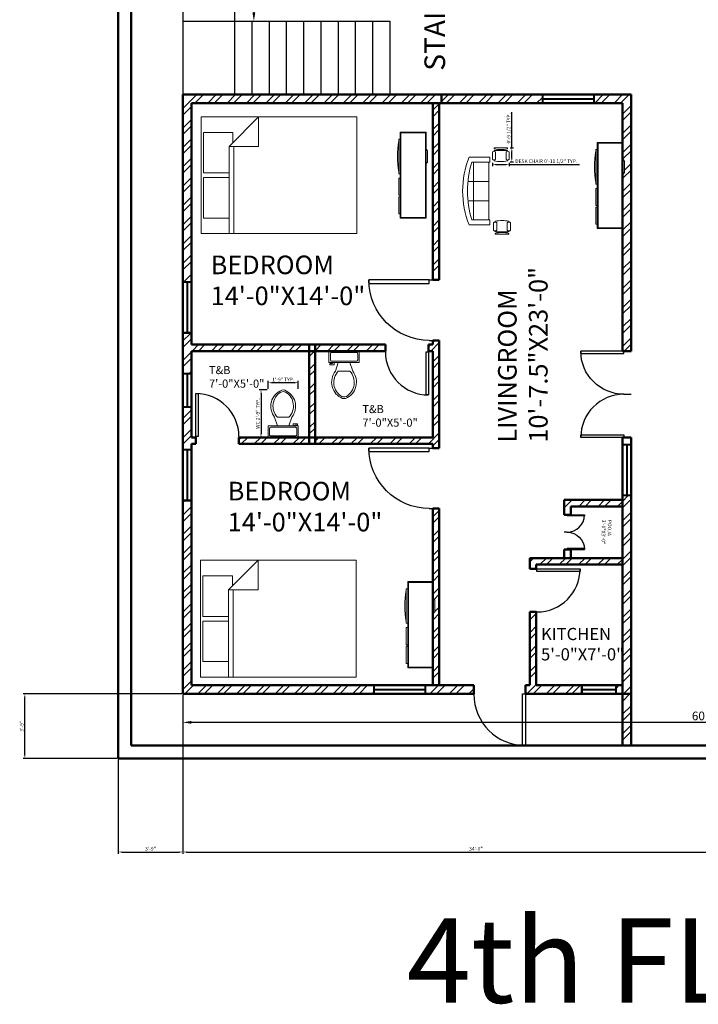
# Model space of a CAD drawing. Units: inches. Extents: x -12550 to 6516, y 1273 to 18700.
# Tile 16 of 19: x 5571 to 6043, y 1273 to 1958. Entities that reach past the tile are written whole.
import ezdxf

# ---------------------------------------------------------------- set-up
doc = ezdxf.new("R2010")
doc.units = ezdxf.units.IN
for name, color, linetype, lineweight in [('A-ANNO-DIMS', 2, 'Continuous', 18), ('A-ANNO-TEXT', 7, 'Continuous', 25), ('A-AREA-IDEN', 1, 'Continuous', 18), ('A-DOOR', 5, 'Continuous', 25), ('A-FLOR-STRS', 6, 'Continuous', 25), ('A-FURN', 8, 'Continuous', 18), ('A-GLAZ', 3, 'Continuous', 25), ('A-WALL', 7, 'Continuous', 50), ('A-WALL-PATT', 8, 'Continuous', 13)]:
    doc.layers.add(name, color=color, linetype=linetype, lineweight=lineweight)
doc.styles.get("Standard").update_dxf_attribs({"font": 'arial.ttf'})
doc.dimstyles.new('ISO-25', dxfattribs={"dimtxt": 2.5, "dimasz": 2.5, "dimexe": 1.25, "dimexo": 0.625, "dimtad": 1, "dimlunit": 4, "dimtxsty": 'Standard', "dimcen": 2.5, "dimadec": 0, "dimazin": 0, "dimtfac": 1, "dimtmove": 0, "dimatfit": 3, "dimfxl": 1, "dimarcsym": 0})
pattern_1 = [(45, (3666.851, 0), (-6.735192, 6.735192), []), (45, (3671.341, 0), (-6.735192, 6.735192), [])]

# ---------------------------------------------------------------- blocks, each defined once
blk = doc.blocks.new('*U2')
for p, q in [((0, 0), (0, -5)), ((30, 0), (30, -5))]:
    blk.add_line(p, q)
blk.add_lwpolyline([(0, 0), (0, 30), (1.75, 30), (1.75, 0)], close=True)
blk.add_arc((0, 0), 30, 0, 90)
blk = doc.blocks.new('Bed - Queen')
for p, q in [((0, -80.00003), (0, 0)), ((0, 0), (59.99999, 0)), ((59.99999, 0), (59.99999, -80.00003)), ((7.99999, -1.2), (28.79998, -1.2)), ((7.99999, -14.4), (7.99999, -1.2)), ((28.79998, -1.2), (28.79998, -14.4)), ((31.19999, -1.2), (51.99999, -1.2)), ((31.19999, -14.4), (31.19999, -1.2)), ((51.99999, -1.2), (51.99999, -16.4)), ((0, -14.4), (44.8, -14.4)), ((59.99999, -29.6), (44.8, -14.4)), ((44.8, -14.4), (44.8, -29.6)), ((44.8, -16.8), (0, -16.8)), ((51.99999, -16.4), (46.79936, -16.4)), ((44.8, -29.6), (59.99999, -29.6)), ((59.99999, -80.00003), (0, -80.00003))]:
    blk.add_line(p, q)
blk = doc.blocks.new('Toilet - top')
for p, q in [((9.5, -6), (9.5, -2)), ((-10, -8.5), (-8, -8.5)), ((-10, -9.5), (-10, -8.5)), ((-7, -9.5), (-10, -9.5)), ((-8, -8.5), (-8, -8)), ((-7, -8), (-7, -9.5)), ((-4, -8), (-6, -14)), ((4, -8), (6, -14)), ((4, -14), (-4, -14))]:
    blk.add_line(p, q)
blk.add_lwpolyline([(10.5, -8), (10.5, 0), (-10.5, 0), (-10.5, -8)], close=True)
for points in [[(-9.5, -2), (-9.5, -6)], [(8.5, -1), (-8.5, -1)], [(-8.5, -7), (8.5, -7)]]:
    blk.add_lwpolyline(points)
for centre, radius, start, end in [((-8.62, -1.88), 0.884, 81.8699, 188.1301), ((-8.62, -6.12), 0.884, 171.8699, 278.1301), ((8.62, -1.88), 0.884, 351.8699, 98.1301), ((8.62, -6.12), 0.884, 261.8699, 8.1301), ((3.52, -21.58), 12.17, 141.46911, 247.97143), ((4.2, -21.82), 11.33, 136.36773, 238.94682), ((-3.52, -21.58), 12.17, 292.02843, 38.53071), ((-4.2, -21.82), 11.33, 301.05301, 43.63209), ((0, -27.88), 4, 245.73182, 294.26817), ((0, -29), 4, 254.86053, 285.13947)]:
    blk.add_arc(centre, radius, start, end)
blk = doc.blocks.new('Entertainment Center')
for p, q in [((-4, 0), (-5, -1)), ((4, 0), (-4, 0)), ((5, -1), (4, 0)), ((-17, -19), (-17, -1)), ((-17, -1), (43, -1)), ((-16.5, -18.5), (-16.5, -1.5)), ((-16.5, -1.5), (42.5, -1.5)), ((42.5, -1.5), (42.5, -18.5)), ((43, -1), (43, -19)), ((43, -19), (-17, -19)), ((42.5, -18.5), (-16.5, -18.5)), ((-12, -20), (-12, -19)), ((12, -20), (-12, -20)), ((12, -19), (12, -20)), ((15, -20), (15, -19)), ((27, -20), (15, -20)), ((27, -19), (27, -20)), ((28, -20), (28, -19)), ((40, -20), (28, -20)), ((40, -19), (40, -20))]:
    blk.add_line(p, q)
blk.add_arc((0, 40), 61, 259.6111, 280.3889)
blk = doc.blocks.new('Sofa - Roundback 7 ft.')
for p, q in [((-36.000027, -34), (-36.000027, -11.4696)), ((-12.00002, -32.4421), (-12.00003, -6.5971)), ((11.99997, -32.4421), (11.99998, -6.5971)), ((35.99998, -34), (35.99998, -11.4696)), ((-35.999844, -13.3819), (35.9998, -13.3819)), ((-36.000027, -32.4421), (35.99998, -32.4421))]:
    blk.add_line(p, q)
for points in [[(-36.000027, -34), (-42.000027, -34), (-42.000027, -8)], [(41.99998, -8), (41.99998, -34), (35.99998, -34)]]:
    blk.add_lwpolyline(points)
for centre, radius, start, end in [((0, -114.25), 114.25, 68.43141, 111.5686), ((-0.00001, -127.1968), 121.1968, 72.72033, 107.2797)]:
    blk.add_arc(centre, radius, start, end)
blk = doc.blocks.new('Chair - Desk')
for p, q in [((-8.5, 0), (-8.5, -1)), ((-8.5, 0), (8.5, 0)), ((8.5, 0), (8.5, -1)), ((-10.5, -5), (-10.5, -14)), ((-8.5, -3), (-8.5, -4)), ((-8.5, -3), (8.5, -3)), ((-6.5, -14), (-6.5, -5)), ((-2, -3), (-2, -1.9355)), ((2, -1.9576), (2, -3)), ((6.5, -5), (6.5, -14)), ((8.5, -3), (8.5, -4)), ((10.5, -14), (10.5, -5)), ((-8.5, -15), (-8.5, -16)), ((8.5, -15), (8.5, -16))]:
    blk.add_line(p, q)
for centre, radius, start, end in [((-8.5, -6.5), 2.5, 36.8699, 143.1301), ((0, 34.625), 36.625, 256.5803, 283.4197), ((8.5, -6.5), 2.5, 36.8699, 143.1301), ((-8.5, -12.5), 2.5, 216.8699, 323.1301), ((0, 19.625), 36.625, 256.5803, 283.4197), ((8.5, -12.5), 2.5, 216.8699, 323.1301)]:
    blk.add_arc(centre, radius, start, end)
blk = doc.blocks.new('*D60')
at = {"layer": 'A-ANNO-DIMS', "color": 0, "lineweight": -2, "transparency": 16777216}
for p, q in [((5721.16, 2008.25), (5735.21, 2008.25)), ((5733.96, 2002.25), (5733.96, 1963.25)), ((5721.16, 1957.25), (5735.21, 1957.25))]:
    blk.add_line(p, q, dxfattribs=at)
at = {"layer": 'A-ANNO-DIMS', "color": 0, "transparency": 16777216}
for points in [[(5732.96, 2002.25), (5734.96, 2002.25), (5733.96, 2008.25)], [(5732.96, 1963.25), (5734.96, 1963.25), (5733.96, 1957.25)]]:
    blk.add_solid(points, dxfattribs=at)
at = {"layer": 'Defpoints', "color": 0, "transparency": 16777216}
for p in [(5720.54, 2008.25), (5720.54, 1957.25), (5733.96, 1957.25)]:
    blk.add_point(p, dxfattribs=at)
at = {"layer": 'A-ANNO-DIMS', "color": 0, "transparency": 16777216, "insert": (5730.27, 1982.75), "char_height": 6, "attachment_point": 5, "rotation": 90}
blk.add_mtext('4\'-3"', dxfattribs=at)
blk = doc.blocks.new('*D55')
at = {"layer": 'A-ANNO-DIMS', "color": 0, "lineweight": -2, "transparency": 16777216}
for p, q in [((5684.54, 1488.62), (5684.54, 1468.21)), ((6404.54, 1488.62), (6404.54, 1468.21)), ((6398.54, 1469.46), (5690.54, 1469.46))]:
    blk.add_line(p, q, dxfattribs=at)
at = {"layer": 'A-ANNO-DIMS', "color": 0, "transparency": 16777216}
for points in [[(5690.54, 1470.46), (5690.54, 1468.46), (5684.54, 1469.46)], [(6398.54, 1470.46), (6398.54, 1468.46), (6404.54, 1469.46)]]:
    blk.add_solid(points, dxfattribs=at)
at = {"layer": 'Defpoints', "color": 0, "transparency": 16777216}
for p in [(5684.54, 1489.25), (6404.54, 1489.25), (5684.54, 1469.46)]:
    blk.add_point(p, dxfattribs=at)
at = {"layer": 'A-ANNO-DIMS', "color": 0, "transparency": 16777216, "insert": (6044.54, 1473.15), "char_height": 6, "attachment_point": 5}
blk.add_mtext("60'", dxfattribs=at)
blk = doc.blocks.new('WIN-3FT')
for p, q in [((0, 0), (0, 6)), ((0, 6), (36.02, 6)), ((36.02, 0), (0, 0)), ((0.5, 0), (0.5, 6)), ((35.52, 3.2), (0.5, 3.2)), ((35.52, 2.8), (0.5, 2.8)), ((35.52, 6), (35.52, 0)), ((36.02, 6), (36.02, 0))]:
    blk.add_line(p, q)
blk = doc.blocks.new('WIN-2FT')
for p, q in [((0, 0), (0, 24.02)), ((0, 24.02), (6, 24.02)), ((0, 23.52), (6, 23.52)), ((2.8, 0.5), (2.8, 23.52)), ((3.2, 0.5), (3.2, 23.52)), ((6, 24.02), (6, 0)), ((6, 0.5), (0, 0.5)), ((6, 0), (0, 0))]:
    blk.add_line(p, q)
blk = doc.blocks.new('*D71')
at = {"layer": 'A-ANNO-DIMS', "color": 0, "lineweight": -2, "transparency": 16777216}
for p, q in [((5743.26, 1700.79), (5737.68, 1700.79)), ((5738.93, 1698.29), (5738.93, 1670.25)), ((5743.26, 1667.75), (5737.68, 1667.75))]:
    blk.add_line(p, q, dxfattribs=at)
at = {"layer": 'A-ANNO-DIMS', "color": 0, "transparency": 16777216}
for points in [[(5738.51, 1698.29), (5739.35, 1698.29), (5738.93, 1700.79)], [(5738.51, 1670.25), (5739.35, 1670.25), (5738.93, 1667.75)]]:
    blk.add_solid(points, dxfattribs=at)
at = {"layer": 'Defpoints', "color": 0, "transparency": 16777216}
for p in [(5743.89, 1700.79), (5738.93, 1667.75), (5743.89, 1667.75)]:
    blk.add_point(p, dxfattribs=at)
at = {"layer": 'A-ANNO-DIMS', "color": 0, "transparency": 16777216, "insert": (5737.01, 1684.27), "char_height": 2.5, "attachment_point": 5, "rotation": 90}
blk.add_mtext('WC 2\'-9" TYP.', dxfattribs=at)
blk = doc.blocks.new('*D72')
at = {"layer": 'A-ANNO-DIMS', "color": 0, "lineweight": -2, "transparency": 16777216}
for p, q in [((5743.89, 1701.42), (5743.89, 1707)), ((5764.89, 1701.42), (5764.89, 1707)), ((5762.39, 1705.75), (5746.39, 1705.75))]:
    blk.add_line(p, q, dxfattribs=at)
at = {"layer": 'A-ANNO-DIMS', "color": 0, "transparency": 16777216}
for points in [[(5746.39, 1706.17), (5746.39, 1705.33), (5743.89, 1705.75)], [(5762.39, 1706.17), (5762.39, 1705.33), (5764.89, 1705.75)]]:
    blk.add_solid(points, dxfattribs=at)
at = {"layer": 'Defpoints', "color": 0, "transparency": 16777216}
for p in [(5743.89, 1705.75), (5743.89, 1700.79), (5764.89, 1700.79)]:
    blk.add_point(p, dxfattribs=at)
at = {"layer": 'A-ANNO-DIMS', "color": 0, "transparency": 16777216, "insert": (5754.39, 1707.65), "char_height": 2.5, "attachment_point": 5}
blk.add_mtext('1\'-9" TYP.', dxfattribs=at)
blk = doc.blocks.new('*D73')
at = {"layer": 'A-ANNO-DIMS', "color": 0, "lineweight": -2, "transparency": 16777216}
for p, q in [((5900.01, 1858.8), (5900.01, 1856.41)), ((5902.51, 1857.66), (5909.26, 1857.66)), ((5911.76, 1858.8), (5911.76, 1856.41)), ((5911.76, 1857.66), (5960.71, 1857.66))]:
    blk.add_line(p, q, dxfattribs=at)
at = {"layer": 'A-ANNO-DIMS', "color": 0, "transparency": 16777216}
for points in [[(5902.51, 1858.08), (5902.51, 1857.24), (5900.01, 1857.66)], [(5909.26, 1858.08), (5909.26, 1857.24), (5911.76, 1857.66)]]:
    blk.add_solid(points, dxfattribs=at)
at = {"layer": 'Defpoints', "color": 0, "transparency": 16777216}
for p in [(5900.01, 1859.42), (5911.76, 1859.42), (5911.76, 1857.66)]:
    blk.add_point(p, dxfattribs=at)
at = {"layer": 'A-ANNO-DIMS', "color": 0, "transparency": 16777216, "insert": (5937.48, 1859.58), "char_height": 2.5, "attachment_point": 5}
blk.add_mtext('DESK CHAIR 0\'-11 1/2" TYP.', dxfattribs=at)
blk = doc.blocks.new('*D74')
at = {"layer": 'A-ANNO-DIMS', "color": 0, "lineweight": -2, "transparency": 16777216}
for p, q in [((5913.52, 1869.12), (5913.52, 1893.94)), ((5912.38, 1869.12), (5914.77, 1869.12)), ((5913.52, 1861.92), (5913.52, 1866.62)), ((5912.38, 1859.42), (5914.77, 1859.42))]:
    blk.add_line(p, q, dxfattribs=at)
at = {"layer": 'A-ANNO-DIMS', "color": 0, "transparency": 16777216}
for points in [[(5913.1, 1866.62), (5913.94, 1866.62), (5913.52, 1869.12)], [(5913.1, 1861.92), (5913.94, 1861.92), (5913.52, 1859.42)]]:
    blk.add_solid(points, dxfattribs=at)
at = {"layer": 'Defpoints', "color": 0, "transparency": 16777216}
for p in [(5911.76, 1869.12), (5913.52, 1869.12), (5911.76, 1859.42)]:
    blk.add_point(p, dxfattribs=at)
at = {"layer": 'A-ANNO-DIMS', "color": 0, "transparency": 16777216, "insert": (5911.6, 1882.78), "char_height": 2.5, "attachment_point": 5, "rotation": 90}
blk.add_mtext('0\'-9 1/2" TYP.', dxfattribs=at)
blk = doc.blocks.new('*D123')
at = {"layer": 'A-ANNO-DIMS', "color": 0, "lineweight": -2, "transparency": 16777216}
for p, q in [((5684.54, 1488.62), (5684.54, 1378)), ((5639.54, 1443.62), (5639.54, 1378)), ((5642.04, 1379.25), (5682.04, 1379.25))]:
    blk.add_line(p, q, dxfattribs=at)
at = {"layer": 'A-ANNO-DIMS', "color": 0, "transparency": 16777216}
for points in [[(5642.04, 1379.66), (5642.04, 1378.83), (5639.54, 1379.25)], [(5682.04, 1379.66), (5682.04, 1378.83), (5684.54, 1379.25)]]:
    blk.add_solid(points, dxfattribs=at)
at = {"layer": 'Defpoints', "color": 0, "transparency": 16777216}
for p in [(5684.54, 1489.25), (5639.54, 1444.25), (5684.54, 1379.25)]:
    blk.add_point(p, dxfattribs=at)
at = {"layer": 'A-ANNO-DIMS', "color": 0, "transparency": 16777216, "insert": (5662.04, 1381.15), "char_height": 2.5, "attachment_point": 5}
blk.add_mtext('3\'-9"', dxfattribs=at)
blk = doc.blocks.new('*D124')
at = {"layer": 'A-ANNO-DIMS', "color": 0, "lineweight": -2, "transparency": 16777216}
for p, q in [((5684.54, 1488.62), (5684.54, 1378)), ((6092.54, 1488.62), (6092.54, 1378)), ((5687.04, 1379.25), (6090.04, 1379.25))]:
    blk.add_line(p, q, dxfattribs=at)
at = {"layer": 'A-ANNO-DIMS', "color": 0, "transparency": 16777216}
for points in [[(5687.04, 1379.66), (5687.04, 1378.83), (5684.54, 1379.25)], [(6090.04, 1379.66), (6090.04, 1378.83), (6092.54, 1379.25)]]:
    blk.add_solid(points, dxfattribs=at)
at = {"layer": 'Defpoints', "color": 0, "transparency": 16777216}
for p in [(5684.54, 1489.25), (6092.54, 1489.25), (6092.54, 1379.25)]:
    blk.add_point(p, dxfattribs=at)
at = {"layer": 'A-ANNO-DIMS', "color": 0, "transparency": 16777216, "insert": (5888.54, 1381.15), "char_height": 2.5, "attachment_point": 5}
blk.add_mtext('34\'-0"', dxfattribs=at)
blk = doc.blocks.new('*D128')
at = {"layer": 'A-ANNO-DIMS', "color": 0, "lineweight": -2, "transparency": 16777216}
for p, q in [((5683.91, 1489.25), (5573.29, 1489.25)), ((5574.54, 1446.75), (5574.54, 1486.75)), ((5638.91, 1444.25), (5573.29, 1444.25))]:
    blk.add_line(p, q, dxfattribs=at)
at = {"layer": 'A-ANNO-DIMS', "color": 0, "transparency": 16777216}
for points in [[(5574.12, 1486.75), (5574.96, 1486.75), (5574.54, 1489.25)], [(5574.12, 1446.75), (5574.96, 1446.75), (5574.54, 1444.25)]]:
    blk.add_solid(points, dxfattribs=at)
at = {"layer": 'Defpoints', "color": 0, "transparency": 16777216}
for p in [(5574.54, 1489.25), (5684.54, 1489.25), (5639.54, 1444.25)]:
    blk.add_point(p, dxfattribs=at)
at = {"layer": 'A-ANNO-DIMS', "color": 0, "transparency": 16777216, "insert": (5572.64, 1466.75), "char_height": 2.5, "attachment_point": 5, "rotation": 90}
blk.add_mtext('3\'-9"', dxfattribs=at)

msp = doc.modelspace()

# ---------------------------------------------------------------- hatches: boundary and pattern name
at = {"layer": 'A-WALL-PATT'}
h = msp.add_hatch(dxfattribs=at)
h.set_pattern_fill('ANSI32', color=256)
h.set_pattern_definition(pattern_1)
h.paths.add_polyline_path([(5690.54, 1900.247), (5864.54, 1900.247), (5864.54, 1906.247), (5684.54, 1906.247), (5684.54, 1776.138), (5690.54, 1776.138)])
h = msp.add_hatch(dxfattribs=at)
h.set_pattern_fill('ANSI32', color=256)
h.set_pattern_definition(pattern_1)
h.paths.add_polyline_path([(5934.791, 1906.247), (5864.54, 1906.247), (5864.54, 1900.247), (5934.791, 1900.247)])
h = msp.add_hatch(dxfattribs=at)
h.set_pattern_fill('ANSI32', color=256)
h.set_pattern_definition(pattern_1)
h.paths.add_polyline_path([(5996.54, 1906.247), (5970.808, 1906.247), (5970.808, 1900.247), (5990.54, 1900.247), (5990.54, 1872.972), (5991.04, 1872.972), (5991.04, 1860.972), (5992.04, 1859.972), (5992.04, 1851.972), (5991.04, 1850.972), (5991.04, 1812.972), (5990.54, 1727.747), (5991.54, 1727.747), (5996.54, 1727.747)])
h = msp.add_hatch(dxfattribs=at)
h.set_pattern_fill('ANSI32', color=256)
h.set_pattern_definition(pattern_1)
h.paths.add_polyline_path([(5863.04, 1900.247), (5858.54, 1900.247), (5858.54, 1777.247), (5863.04, 1777.247)], flags=17)
h = msp.add_hatch(dxfattribs=at)
h.set_pattern_fill('ANSI32', color=256)
h.set_pattern_definition(pattern_1)
h.paths.add_polyline_path([(5772.54, 1732.247), (5690.54, 1732.247), (5690.54, 1740.121), (5684.54, 1740.121), (5684.54, 1712.466), (5690.54, 1712.466), (5690.54, 1727.747), (5772.54, 1727.747)])
h = msp.add_hatch(dxfattribs=at)
h.set_pattern_fill('ANSI32', color=256)
h.set_pattern_definition(pattern_1)
h.paths.add_polyline_path([(5863.04, 1735.247), (5858.54, 1735.247), (5858.54, 1732.247), (5855.54, 1732.247), (5855.54, 1727.747), (5858.54, 1727.747), (5858.54, 1667.747), (5776.54, 1667.747), (5776.54, 1663.247), (5858.54, 1663.247), (5858.54, 1660.247), (5863.04, 1660.247)])
h = msp.add_hatch(dxfattribs=at)
h.set_pattern_fill('ANSI32', color=256)
h.set_pattern_definition(pattern_1)
h.paths.add_polyline_path([(5776.54, 1727.747), (5772.54, 1727.747), (5772.54, 1667.747), (5776.54, 1667.747)])
h = msp.add_hatch(dxfattribs=at)
h.set_pattern_fill('ANSI32', color=256)
h.set_pattern_definition(pattern_1)
h.paths.add_polyline_path([(5825.54, 1732.247), (5776.54, 1732.247), (5776.54, 1727.747), (5825.54, 1727.747)], flags=17)
h = msp.add_hatch(dxfattribs=at)
h.set_pattern_fill('ANSI32', color=256)
h.set_pattern_definition(pattern_1)
h.paths.add_polyline_path([(5690.54, 1688.449), (5684.54, 1688.449), (5684.54, 1659.453), (5690.54, 1659.453), (5690.54, 1663.247), (5693.54, 1663.247), (5693.54, 1667.747), (5690.54, 1667.747)])
h = msp.add_hatch(dxfattribs=at)
h.set_pattern_fill('ANSI32', color=256)
h.set_pattern_definition(pattern_1)
h.paths.add_polyline_path([(5772.54, 1667.747), (5723.54, 1667.747), (5723.54, 1663.247), (5772.54, 1663.247)])
h = msp.add_hatch(dxfattribs=at)
h.set_pattern_fill('ANSI32', color=256)
h.set_pattern_definition(pattern_1)
h.paths.add_polyline_path([(5990.54, 1624.247), (5950.04, 1624.247), (5950.04, 1613.747), (5952.04, 1613.747), (5954.54, 1613.747), (5954.54, 1619.747), (5990.54, 1619.747)])
h = msp.add_hatch(dxfattribs=at)
h.set_pattern_fill('ANSI32', color=256)
h.set_pattern_definition(pattern_1)
h.paths.add_polyline_path([(5996.54, 1627.032), (5990.54, 1627.032), (5990.54, 1495.247), (5986.145, 1495.247), (5986.145, 1489.247), (5996.54, 1489.247)])
h = msp.add_hatch(dxfattribs=at)
h.set_pattern_fill('ANSI32', color=256)
h.set_pattern_definition(pattern_1)
h.paths.add_polyline_path([(5690.54, 1623.435), (5684.54, 1623.435), (5684.54, 1489.247), (5817.49, 1489.247), (5817.49, 1495.247), (5690.54, 1495.247)])
h = msp.add_hatch(dxfattribs=at)
h.set_pattern_fill('ANSI32', color=256)
h.set_pattern_definition(pattern_1)
h.paths.add_polyline_path([(5863.04, 1618.247), (5858.54, 1618.247), (5858.54, 1567.365), (5859.04, 1567.365), (5859.04, 1555.365), (5860.04, 1554.365), (5860.04, 1546.365), (5859.04, 1545.365), (5859.04, 1507.365), (5858.54, 1495.247), (5863.04, 1495.247)])
h = msp.add_hatch(dxfattribs=at)
h.set_pattern_fill('ANSI32', color=256)
h.set_pattern_definition(pattern_1)
h.paths.add_polyline_path([(5990.54, 1583.747), (5926.04, 1583.747), (5926.04, 1576.247), (5930.54, 1576.247), (5930.54, 1579.247), (5990.54, 1579.247)])
h = msp.add_hatch(dxfattribs=at)
h.set_pattern_fill('ANSI32', color=256)
h.set_pattern_definition(pattern_1)
h.paths.add_polyline_path([(5962.127, 1495.247), (5930.54, 1495.247), (5930.54, 1546.247), (5926.04, 1546.247), (5926.04, 1495.247), (5923.04, 1495.247), (5923.04, 1489.247), (5962.127, 1489.247)])
h = msp.add_hatch(dxfattribs=at)
h.set_pattern_fill('ANSI32', color=256)
h.set_pattern_definition(pattern_1)
h.paths.add_polyline_path([(5887.04, 1495.247), (5853.508, 1495.247), (5853.508, 1489.247), (5887.04, 1489.247)])
h = msp.add_hatch(dxfattribs=at)
h.set_pattern_fill('ANSI32', color=256)
h.set_pattern_definition(pattern_1)
h.paths.add_polyline_path([(5996.54, 1489.247), (5990.54, 1489.247), (5990.54, 1453.247), (5996.54, 1453.247)])

# ---------------------------------------------------------------- linework, layer by layer
at = {"layer": 'A-FLOR-STRS'}
for p, q in [((5684.54, 2056.247), (5684.54, 1906.247)), ((5720.54, 2056.247), (5720.54, 1906.247)), ((5684.54, 1957.247), (5828.54, 1957.247)), ((5732.54, 1957.247), (5732.54, 1906.247)), ((5744.54, 1957.247), (5744.54, 1906.247)), ((5756.54, 1957.247), (5756.54, 1906.247)), ((5768.54, 1957.247), (5768.54, 1906.247)), ((5780.54, 1957.247), (5780.54, 1906.247)), ((5792.54, 1957.247), (5792.54, 1906.247)), ((5804.54, 1957.247), (5804.54, 1906.247)), ((5816.54, 1957.247), (5816.54, 1906.247)), ((5828.54, 1957.247), (5828.54, 1906.247)), ((5684.54, 1906.247), (5864.54, 1906.247))]:
    msp.add_line(p, q, dxfattribs=at)
at = {"layer": 'A-WALL'}
for p, q in [((5639.54, 1444.247), (5639.54, 2518.247)), ((5648.54, 1453.247), (5648.54, 2509.247)), ((5996.54, 1906.247), (5684.54, 1906.247)), ((5684.54, 1489.247), (5684.54, 1906.247)), ((5864.54, 1900.247), (5864.54, 1906.247)), ((5996.54, 1727.747), (5996.54, 1906.247)), ((5990.54, 1900.247), (5690.54, 1900.247)), ((5690.54, 1732.247), (5690.54, 1900.247)), ((5858.54, 1777.247), (5858.54, 1900.247)), ((5863.04, 1777.247), (5863.04, 1900.247)), ((5990.54, 1727.747), (5990.54, 1900.247)), ((5863.04, 1777.247), (5858.54, 1777.247)), ((5858.54, 1732.247), (5858.54, 1735.247)), ((5858.54, 1732.247), (5858.54, 1735.247)), ((5858.54, 1735.247), (5863.04, 1735.247)), ((5863.04, 1660.247), (5863.04, 1735.247)), ((5825.54, 1732.247), (5690.54, 1732.247)), ((5825.54, 1727.747), (5690.54, 1727.747)), ((5690.54, 1667.747), (5690.54, 1727.747)), ((5772.54, 1663.247), (5772.54, 1732.247)), ((5776.54, 1663.247), (5776.54, 1732.247)), ((5825.54, 1727.747), (5825.54, 1732.247)), ((5858.54, 1732.247), (5855.54, 1732.247)), ((5858.54, 1732.247), (5855.54, 1732.247)), ((5855.54, 1732.247), (5855.54, 1727.747)), ((5858.54, 1727.747), (5855.54, 1727.747)), ((5858.54, 1667.747), (5858.54, 1727.747)), ((5996.54, 1727.747), (5990.54, 1727.747)), ((5693.54, 1667.747), (5690.54, 1667.747)), ((5693.54, 1663.247), (5693.54, 1667.747)), ((5858.54, 1667.747), (5723.54, 1667.747)), ((5723.54, 1667.747), (5858.54, 1667.747)), ((5723.54, 1667.747), (5723.54, 1663.247)), ((5996.54, 1667.747), (5990.54, 1667.747)), ((5990.54, 1453.247), (5990.54, 1667.747)), ((5996.54, 1489.247), (5996.54, 1667.747)), ((5693.54, 1663.247), (5690.54, 1663.247)), ((5690.54, 1495.247), (5690.54, 1663.247)), ((5690.54, 1663.247), (5693.54, 1663.247)), ((5858.54, 1663.247), (5723.54, 1663.247)), ((5858.54, 1660.247), (5858.54, 1663.247)), ((5863.04, 1660.247), (5858.54, 1660.247)), ((5863.04, 1663.247), (5863.04, 1660.247)), ((5990.54, 1624.247), (5950.04, 1624.247)), ((5950.04, 1613.747), (5950.04, 1624.247)), ((5858.54, 1495.247), (5858.54, 1618.247)), ((5858.54, 1618.247), (5863.04, 1618.247)), ((5863.04, 1495.247), (5863.04, 1618.247)), ((5990.54, 1619.747), (5954.54, 1619.747)), ((5954.54, 1613.747), (5954.54, 1619.747)), ((5950.04, 1613.747), (5954.54, 1613.747)), ((5950.04, 1583.747), (5950.04, 1589.747)), ((5954.54, 1589.747), (5950.04, 1589.747)), ((5954.54, 1583.747), (5954.54, 1589.747)), ((5954.54, 1583.747), (5954.54, 1589.747)), ((5990.54, 1583.747), (5926.04, 1583.747)), ((5926.04, 1576.247), (5926.04, 1583.747)), ((5950.04, 1583.747), (5950.04, 1588.747)), ((5930.54, 1576.247), (5926.04, 1576.247)), ((5990.54, 1579.247), (5930.54, 1579.247)), ((5930.54, 1576.247), (5930.54, 1579.247)), ((5930.54, 1579.247), (5930.54, 1576.247)), ((5926.04, 1495.247), (5926.04, 1546.247)), ((5926.04, 1546.247), (5930.54, 1546.247)), ((5930.54, 1495.247), (5930.54, 1546.247)), ((5887.04, 1495.247), (5690.54, 1495.247)), ((5887.04, 1495.247), (5863.04, 1495.247)), ((5887.04, 1489.247), (5887.04, 1495.247)), ((5926.04, 1495.247), (5923.04, 1495.247)), ((5926.04, 1495.247), (5923.04, 1495.247)), ((5923.04, 1495.247), (5923.04, 1489.247)), ((5990.54, 1495.247), (5930.54, 1495.247)), ((5887.04, 1489.247), (5684.54, 1489.247)), ((5996.54, 1489.247), (5923.04, 1489.247)), ((5996.54, 1489.247), (5996.54, 1453.247)), ((5648.54, 1453.247), (6440.54, 1453.247)), ((6187.04, 1453.247), (5923.04, 1453.247)), ((5639.54, 1444.247), (6449.54, 1444.247))]:
    msp.add_line(p, q, dxfattribs=at)

# ---------------------------------------------------------------- block references
at = {"layer": 'A-DOOR'}
for p, xscale, yscale, zscale, rotation in [((5856.04, 1777.247), -1.4, 1.4, 1.4, 90), ((5856.04, 1660.247), -1.4, 1.4, 1.4, 90), ((5952.04, 1613.747), 0.399999999999997, 0.399999999999997, 0.399999999999997, 270), ((5952.04, 1589.747), -0.399999999999997, 0.399999999999997, 0.399999999999997, 270), ((5923.04, 1489.247), 1.199999999999999, 1.199999999999999, 1.199999999999999, 180)]:
    msp.add_blockref('*U2', p, dxfattribs=dict(at, xscale=xscale, yscale=yscale, zscale=zscale, rotation=rotation))
for p, rotation in [((5855.54, 1727.247), 180), ((5991.54, 1667.747), 90), ((5931.04, 1576.247), 270)]:
    msp.add_blockref('*U2', p, dxfattribs=dict(at, rotation=rotation))
at = {"layer": 'A-DOOR', "xscale": -1, "rotation": 90}
msp.add_blockref('*U2', (5991.54, 1727.747), dxfattribs=at)
at = {"layer": 'A-DOOR'}
msp.add_blockref('*U2', (5693.54, 1668.247), dxfattribs=at)
at = {"layer": 'A-FURN'}
for name, p, xscale, yscale, zscale, rotation in [('Bed - Queen', (5697.19, 1809.493), 1.354827908062564, 1.354827908062564, 1.354827908062564, 90), ('Sofa - Roundback 7 ft.', (5879.299, 1839.138), 0.5595223685495907, 0.5595223685495907, 0.5595223685495907, 90), ('Chair - Desk', (5906.738, 1809.138), 0.5595223685495907, 0.5595223685495907, 0.5595223685495907, 180), ('Bed - Queen', (5696.888, 1500.915), 1.354827908062564, 1.354827908062564, 1.354827908062564, 90)]:
    msp.add_blockref(name, p, dxfattribs=dict(at, xscale=xscale, yscale=yscale, zscale=zscale, rotation=rotation))
for name, p, rotation in [('Entertainment Center', (5854.881, 1863.204), 270), ('Entertainment Center', (5992.04, 1855.972), 270), ('Toilet - top', (5754.387, 1667.747), 180), ('Entertainment Center', (5860.04, 1550.365), 270)]:
    msp.add_blockref(name, p, dxfattribs=dict(at, rotation=rotation))
at = {"layer": 'A-FURN', "xscale": 0.5595223685495907, "yscale": 0.5595223685495907, "zscale": 0.5595223685495907}
msp.add_blockref('Chair - Desk', (5905.884, 1869.122), dxfattribs=at)
at = {"layer": 'A-FURN'}
msp.add_blockref('Toilet - top', (5796.751, 1727.747), dxfattribs=at)
at = {"layer": 'A-GLAZ'}
for name, p, rotation in [('WIN-3FT', (5970.808, 1906.247), 180), ('WIN-3FT', (5690.54, 1740.121), 90.00000000000458), ('WIN-2FT', (5690.539, 1712.467), 180), ('WIN-3FT', (5690.54, 1623.436), 90.00000000000445), ('WIN-3FT', (5996.54, 1627.032), 89.9999999999992), ('WIN-3FT', (5853.508, 1495.247), 180), ('WIN-2FT', (5962.127, 1495.247), 269.9999999999944)]:
    msp.add_blockref(name, p, dxfattribs=dict(at, rotation=rotation))

# ---------------------------------------------------------------- texts
at = {"layer": 'A-ANNO-TEXT', "insert": (5840.46, 1333.138), "char_height": 58.816, "attachment_point": 1}
msp.add_mtext('4th FLOOR', dxfattribs=at)
at = {"layer": 'A-AREA-IDEN', "attachment_point": 1}
for s, width, gutter_width, insert, char_height, rotation in [('STAIRCASE', 2.19144, 71.795, (5852.716, 1922.837), 14.3589, 90), ('POOJA\\P3\'-0"X3\'-0"', 0.78585, 12.5, (5982.916, 1610.304), 2.5, 269.183853)]:
    msp.add_mtext_dynamic_manual_height_columns(s, width=width, gutter_width=gutter_width, heights=[0], dxfattribs=dict(at, insert=insert, char_height=char_height, rotation=rotation))
at = {"layer": 'A-AREA-IDEN', "char_height": 12.93169, "attachment_point": 1}
for insert in [(5703.876, 1794.217), (5715.757, 1636.812)]:
    msp.add_mtext('BEDROOM\\P14\'-0"X14\'-0"', dxfattribs=dict(at, insert=insert))
at = {"layer": 'A-AREA-IDEN', "insert": (5903.946, 1664.034), "char_height": 12.93169, "attachment_point": 1, "rotation": 90}
msp.add_mtext('LIVINGROOM\\P10\'-7.5"X23\'-0"', dxfattribs=at)
at = {"layer": 'A-AREA-IDEN', "attachment_point": 1}
for s, width, gutter_width, insert, char_height in [('T&B\\P7\'-0"X5\'-0"', 4.19569, 28.328, (5702.715, 1717.416), 5.66556), ('T&B\\P7\'-0"X5\'-0"', 4.19569, 28.328, (5809.477, 1690.282), 5.66556), ('KITCHEN\\P5\'-0"X7\'-0"', 1.29487, 42.422, (5933.861, 1535.176), 8.48435)]:
    msp.add_mtext_dynamic_manual_height_columns(s, width=width, gutter_width=gutter_width, heights=[0], dxfattribs=dict(at, insert=insert, char_height=char_height))

# ---------------------------------------------------------------- dimensions: what is measured, and where the dimension line sits
at = {"layer": 'A-ANNO-DIMS'}
for base, p1, p2, override, picture, middle in [((5733.962, 1957.247), (5720.54, 2008.247), (5720.54, 1957.247), {"dimtxt": 6, "dimasz": 6, "dimclrd": 0, "dimclre": 0, "dimclrt": 0}, '*D60', (5730.271, 1982.747)), ((5574.54, 1489.247), (5639.54, 1444.247), (5684.54, 1489.247), {"dimdec": 1, "dimlfac": 1, "dimrnd": 0, "dimzin": 1, "dimdsep": 46, "dimlunit": 4, "dimfrac": 2}, '*D128', (5572.637, 1466.747))]:
    dim = msp.add_linear_dim(base=base, p1=p1, p2=p2, angle=90, dimstyle='ISO-25', override=override, dxfattribs=at)
    dim.commit()
    dim.dimension.update_dxf_attribs({"geometry": picture, "text_midpoint": middle})
for base, p1, p2, angle, text, picture, middle in [((5913.522, 1869.122), (5911.759, 1859.424), (5911.759, 1869.122), 90, '<> TYP.', '*D74', (5911.604, 1882.779)), ((5743.887, 1705.75), (5764.887, 1700.793), (5743.887, 1700.793), 180, '<> TYP.', '*D72', (5754.387, 1707.652)), ((5738.93, 1667.747), (5743.887, 1700.793), (5743.887, 1667.747), 270, 'WC <> TYP.', '*D71', (5737.012, 1684.27))]:
    dim = msp.add_linear_dim(base=base, p1=p1, p2=p2, angle=angle, text=text, dimstyle='ISO-25', override={"dimdec": 1, "dimrnd": 0, "dimzin": 1, "dimlunit": 4, "dimfrac": 2}, dxfattribs=at)
    dim.commit()
    dim.dimension.update_dxf_attribs({"geometry": picture, "text_midpoint": middle})
dim = msp.add_linear_dim(base=(5911.75906, 1857.6611), p1=(5900.00909, 1859.42359), p2=(5911.75906, 1859.42359), text='DESK CHAIR <> TYP.', dimstyle='ISO-25', override={"dimdec": 1, "dimrnd": 0, "dimzin": 1, "dimlunit": 4, "dimfrac": 2}, dxfattribs=at)
dim.commit()
dim.dimension.update_dxf_attribs({"geometry": '*D73', "text_midpoint": (5937.48382, 1859.57873)})
for base, p1, p2, override, picture, middle in [((5684.54, 1379.247), (5639.54, 1444.247), (5684.54, 1489.247), {"dimdec": 1, "dimlfac": 1, "dimrnd": 0, "dimzin": 1, "dimdsep": 46, "dimlunit": 4, "dimfrac": 2}, '*D123', (5662.04, 1381.15)), ((5684.54, 1469.461), (6404.54, 1489.247), (5684.54, 1489.247), {"dimtxt": 6, "dimasz": 6, "dimclrd": 0, "dimclre": 0, "dimclrt": 0}, '*D55', (6044.54, 1473.15)), ((6092.54, 1379.247), (5684.54, 1489.247), (6092.54, 1489.247), {"dimdec": 1, "dimlfac": 1, "dimrnd": 0, "dimzin": 1, "dimdsep": 46, "dimlunit": 4, "dimfrac": 2}, '*D124', (5888.54, 1381.15))]:
    dim = msp.add_linear_dim(base=base, p1=p1, p2=p2, dimstyle='ISO-25', override=override, dxfattribs=at)
    dim.commit()
    dim.dimension.update_dxf_attribs({"geometry": picture, "text_midpoint": middle})

doc.saveas('drawing.dxf')
